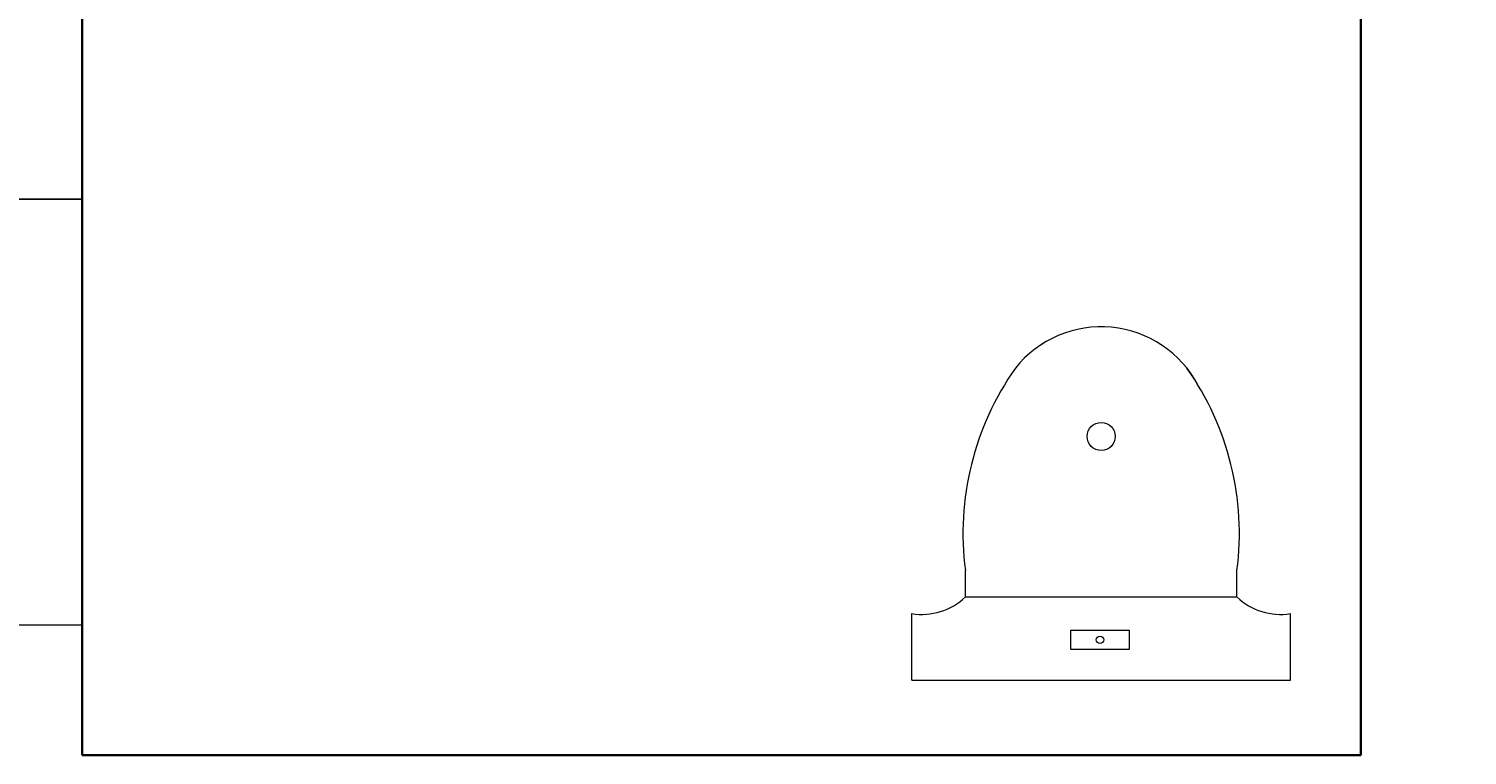
# Model space of a CAD drawing. Units: inches. Extents: x -61 to 1599, y -1316 to 257.
# Tile 60 of 204: x 85 to 166, y -282 to -241. Entities that reach past the tile are written whole.
import ezdxf

# ---------------------------------------------------------------- set-up
doc = ezdxf.new("R2010")
doc.units = ezdxf.units.IN
doc.header["$MEASUREMENT"] = 0
for name, color, linetype, lineweight in [('A-ANNO-DIMS', 2, 'Continuous', 18), ('A-FLOR-FIXT', 8, 'Continuous', 18), ('WALLS', 4, 'Continuous', 35), ('WINDOWS', 220, 'Continuous', 18)]:
    doc.layers.add(name, color=color, linetype=linetype, lineweight=lineweight)
doc.styles.get("Standard").update_dxf_attribs({"font": 'arial.ttf'})
doc.dimstyles.get("Standard").update_dxf_attribs({"dimtxt": 0.18, "dimasz": 0.18, "dimexe": 0.18, "dimexo": 0.0625, "dimgap": 0.09, "dimtad": 0, "dimtih": 1, "dimtoh": 1, "dimdec": 0, "dimzin": 0, "dimdsep": 46, "dimlunit": 3, "dimtxsty": 'Standard', "dimcen": 0.09, "dimadec": 0, "dimazin": 0, "dimtfac": 1, "dimtdec": 0, "dimtofl": 0, "dimtmove": 0, "dimatfit": 3, "dimfxl": 1, "dimtolj": 1, "dimtzin": 0, "dimarcsym": 0})

# ---------------------------------------------------------------- blocks, each defined once
blk = doc.blocks.new('WIN-24IN')
for p, q in [((0, 4.5), (0, 9)), ((0, 9), (0, 0)), ((24, 9), (24, 0)), ((0, 5.192), (24, 5.192)), ((0, 4.5), (24, 4.5))]:
    blk.add_line(p, q)
blk = doc.blocks.new('WC-FLOOR-MOUNT')
for p, q in [((3.018, 4.686), (3.018, 6.173)), ((18.314, 4.686), (18.314, 6.173)), ((3.018, 4.686), (18.314, 4.686)), ((0, 0), (0, 3.747)), ((21.331, 0), (21.331, 3.747)), ((0, 0), (21.331, 0))]:
    blk.add_line(p, q)
blk.add_lwpolyline([(12.243, 1.734), (8.955, 1.734), (8.955, 2.812), (12.243, 2.812)], close=True)
for centre, radius in [((10.666, 13.729), 0.792), ((10.599, 2.273), 0.208)]:
    blk.add_circle(centre, radius)
for centre, radius, start, end in [((10.666, 13.729), 6.176, 27.68441, 141.46969), ((19.051, 8.262), 16.169, 144.82396, 187.42318), ((2.281, 8.262), 16.169, 352.57682, 35.17604), ((0.565, 7.253), 3.551, 260.8586, 313.6993), ((20.767, 7.253), 3.551, 226.3007, 279.1414)]:
    blk.add_arc(centre, radius, start, end)
blk = doc.blocks.new('*D687')
at = {"layer": 'A-ANNO-DIMS', "color": 0, "lineweight": -2, "transparency": 16777216}
for p, q in [((289.418, 181.677), (-61.077, 181.677)), ((-60.897, 181.497), (-60.897, -528.952)), ((-60.897, -1239.765), (-60.897, -529.316)), ((319.64, -1239.945), (-61.077, -1239.945))]:
    blk.add_line(p, q, dxfattribs=at)
at = {"layer": 'A-ANNO-DIMS', "color": 0, "transparency": 16777216}
for points in [[(-60.927, 181.497), (-60.867, 181.497), (-60.897, 181.677)], [(-60.927, -1239.765), (-60.867, -1239.765), (-60.897, -1239.945)]]:
    blk.add_solid(points, dxfattribs=at)
at = {"layer": 'DEFPOINTS', "color": 0, "transparency": 16777216}
for p in [(289.481, 181.677), (-60.897, -1239.945), (319.703, -1239.945)]:
    blk.add_point(p, dxfattribs=at)
at = {"layer": 'A-ANNO-DIMS', "color": 0, "transparency": 16777216, "insert": (-60.897, -529.134), "char_height": 0.18, "attachment_point": 5}
blk.add_mtext('\\A1;1421.6', dxfattribs=at)
blk = doc.blocks.new('*D699')
at = {"layer": 'A-ANNO-DIMS', "color": 0, "lineweight": -2, "transparency": 16777216}
for p, q in [((835.64, -167.169), (-61.077, -167.169)), ((-60.897, -167.349), (-60.897, -306.726)), ((-60.897, -446.466), (-60.897, -307.09)), ((841.64, -446.646), (-61.077, -446.646))]:
    blk.add_line(p, q, dxfattribs=at)
at = {"layer": 'A-ANNO-DIMS', "color": 0, "transparency": 16777216}
for points in [[(-60.927, -167.349), (-60.867, -167.349), (-60.897, -167.169)], [(-60.927, -446.466), (-60.867, -446.466), (-60.897, -446.646)]]:
    blk.add_solid(points, dxfattribs=at)
at = {"layer": 'DEFPOINTS', "color": 0, "transparency": 16777216}
for p in [(835.703, -167.169), (-60.897, -446.646), (841.703, -446.646)]:
    blk.add_point(p, dxfattribs=at)
at = {"layer": 'A-ANNO-DIMS', "color": 0, "transparency": 16777216, "insert": (-60.897, -306.908), "char_height": 0.18, "attachment_point": 5}
blk.add_mtext('\\A1;279.5', dxfattribs=at)
blk = doc.blocks.new('*D700')
at = {"layer": 'A-ANNO-DIMS', "color": 0, "lineweight": -2, "transparency": 16777216}
for p, q in [((14.703, -616.882), (14.703, 257.457)), ((14.883, 257.277), (96.772, 257.277)), ((179.572, 257.277), (97.683, 257.277)), ((179.752, -616.882), (179.752, 257.457))]:
    blk.add_line(p, q, dxfattribs=at)
at = {"layer": 'A-ANNO-DIMS', "color": 0, "transparency": 16777216}
for points in [[(14.883, 257.307), (14.883, 257.247), (14.703, 257.277)], [(179.572, 257.307), (179.572, 257.247), (179.752, 257.277)]]:
    blk.add_solid(points, dxfattribs=at)
at = {"layer": 'DEFPOINTS', "color": 0, "transparency": 16777216}
for p in [(179.752, 257.277), (14.703, -616.945), (179.752, -616.945)]:
    blk.add_point(p, dxfattribs=at)
at = {"layer": 'A-ANNO-DIMS', "color": 0, "transparency": 16777216, "insert": (97.227, 257.277), "char_height": 0.18, "attachment_point": 5}
blk.add_mtext('\\A1;165.05', dxfattribs=at)

msp = doc.modelspace()

# ---------------------------------------------------------------- linework, layer by layer
at = {"layer": 'WALLS'}
for p, q in [((87.7028, -282.3229), (87.7028, -175.3229)), ((159.7028, -282.3229), (159.7028, -175.3229)), ((87.7028, -282.3229), (159.7028, -282.3229))]:
    msp.add_line(p, q, dxfattribs=at)

# ---------------------------------------------------------------- block references
at = {"layer": 'A-FLOR-FIXT'}
msp.add_blockref('WC-FLOOR-MOUNT', (134.4199, -278.0925), dxfattribs=at)
at = {"layer": 'WINDOWS', "rotation": 270.0000000000001}
msp.add_blockref('WIN-24IN', (78.7027, -250.9933), dxfattribs=at)

# ---------------------------------------------------------------- dimensions: what is measured, and where the dimension line sits
at = {"layer": 'A-ANNO-DIMS'}
dim = msp.add_linear_dim(base=(179.7521, 257.2771), p1=(14.7028, -616.9446), p2=(179.7521, -616.9446), dimstyle='Standard', override={"dimdec": 2, "dimlfac": 1, "dimrnd": 0, "dimzin": 0, "dimdsep": 46, "dimlunit": 2}, dxfattribs=at)
dim.commit()
dim.dimension.update_dxf_attribs({"geometry": '*D700', "text_midpoint": (97.2274, 257.2771)})
for base, p1, p2, picture, middle in [((-60.8972, -1239.9446), (289.4807, 181.6771), (319.7028, -1239.9446), '*D687', (-60.8972, -529.1337)), ((-60.8972, -446.6462), (835.7028, -167.169), (841.7028, -446.6462), '*D699', (-60.8972, -306.9076))]:
    dim = msp.add_linear_dim(base=base, p1=p1, p2=p2, angle=90, dimstyle='Standard', override={"dimdec": 1, "dimlfac": 1, "dimrnd": 0, "dimzin": 0, "dimdsep": 46, "dimlunit": 2}, dxfattribs=at)
    dim.commit()
    dim.dimension.update_dxf_attribs({"geometry": picture, "text_midpoint": middle})

doc.saveas('drawing.dxf')
